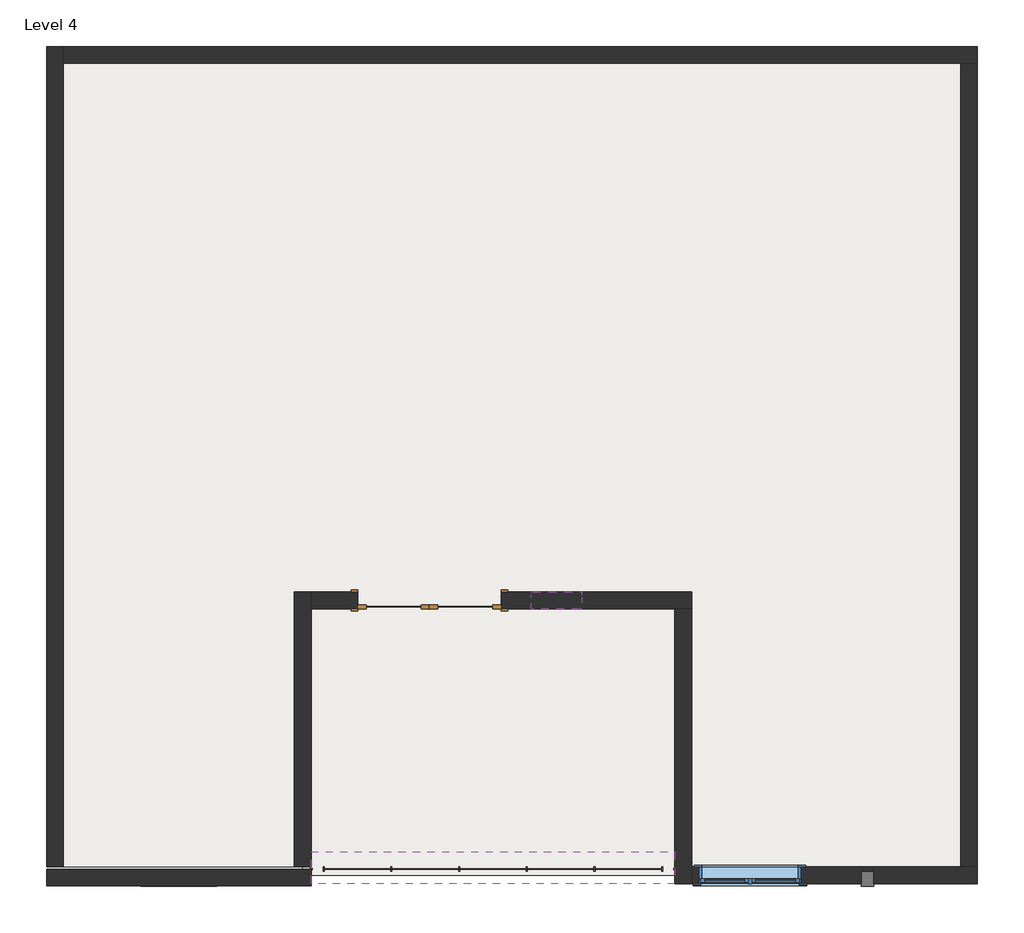
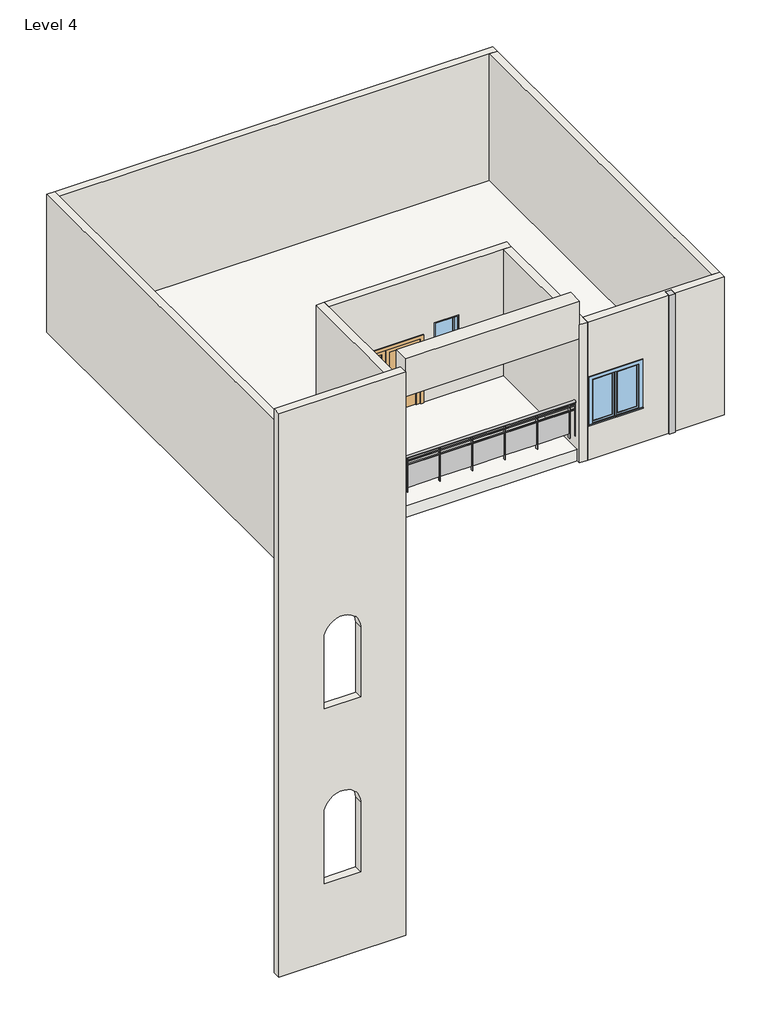
# One storey: 9 walls, 2 windows, 1 door, 1 proxy, 1 railing, 1 roof.
"""IFC4 building model written with IfcOpenShell, lengths in millimetres."""

from ifc_helpers import new_model, si_unit, point, frame, frame_2d, origin, place, context, project, spatial, polyline, circle_curve, ellipse_curve, trimmed, segment, composite_curve, outline, extrude, faceted_brep, transform, mapped, element, save
from ifc_brep_helpers import plane_surface, extruded_surface, advanced_brep
from components import door_10418eaf, walls_3_walls_2_f167fe74, window_0862ab64, window_6846e476

model = new_model("IFC4")

# Units and contexts
model_context = context("Model", 3, world=origin())
ifc_project = project(units=[si_unit("LENGTHUNIT", "METRE", prefix="MILLI")], contexts=[model_context])

# Site, building, storey
site = spatial("IfcSite", under=ifc_project)
building = spatial("IfcBuilding", under=site)
storey = spatial("IfcBuildingStorey", under=building, Name="Level 4", Elevation=10972.8)

# Proxy
placement = place(None, origin())
element("IfcBuildingElementProxy", 1, Name="Reveal", ObjectType="Reveal", at=placement, inside=storey, context=model_context, shape_type="SweptSolid", body=[
    extrude(outline(polyline([(752.5001186, 242.2810824), (752.5001186, 425.1610824), (904.9001186, 425.1610824), (904.9001186, 242.2810824), (752.5001186, 242.2810824)])), frame((0.0, 0.0, 10972.8), z_axis=(0.0, 0.0, 1.0), x_axis=(1.0, 0.0, 0.0)), (0.0, 0.0, 1.0), 3657.6),
])

# Door
door_shape = door_10418eaf(model_context)
element("IfcDoor", 2, ObjectType="Door-Double-Glass : 68\" x 80\"", at=placement, inside=storey, context=model_context, shape_type="MappedRepresentation", body=[
    mapped(door_shape, transform((-4429.0998814, 3678.7423324, 10972.8), x_axis=(-1.0, 0.0, 0.0), y_axis=(0.0, -1.0, 0.0), z_axis=(0.0, 0.0, 1.0))),
])

# Railing
element("IfcRailing", 3, ObjectType="Glass Panel - Bottom Fill", at=placement, inside=storey, context=model_context, shape_type="SolidModel", body=[
    advanced_brep(
    [(-5851.4998814, 488.6610824, 12496.8), (-5851.4998814, 412.4610824, 12496.8), (-1482.6998814, 488.6610824, 12496.8), (-1482.6998814, 412.4610824, 12496.8)],
    [
        (0, 1, ellipse_curve(frame((-5851.4998814, 450.5610824, 12496.8), z_axis=(-1.0, 0.0, 0.0), x_axis=(0.0, -1.0, 0.0)), 38.1, 28.575)),
        (1, 0, ellipse_curve(frame((-5851.4998814, 450.5610824, 12496.8), z_axis=(-1.0, 0.0, 0.0), x_axis=(0.0, -1.0, 0.0)), 38.1, 28.575)),
        (2, 3, ellipse_curve(frame((-1482.6998814, 450.5610824, 12496.8), z_axis=(1.0, 0.0, 0.0), x_axis=(0.0, -1.0, 0.0)), 38.1, 28.575)),
        (3, 2, ellipse_curve(frame((-1482.6998814, 450.5610824, 12496.8), z_axis=(1.0, 0.0, 0.0), x_axis=(0.0, -1.0, 0.0)), 38.1, 28.575)),
        (0, 2),
        (3, 1),
    ],
    [
        plane_surface(frame((-5851.4998814, 450.5610824, 12496.8), z_axis=(-1.0, 0.0, 0.0), x_axis=(0.0, 1.0, 0.0))),
        plane_surface(frame((-1482.6998814, 450.5610824, 12496.8), z_axis=(1.0, 0.0, 0.0), x_axis=(0.0, 1.0, 0.0))),
        extruded_surface(trimmed(ellipse_curve(frame((-1482.6998814, 450.5610824, 12496.8), z_axis=(-1.0, 0.0, 0.0), x_axis=(0.0, -1.0, 0.0)), 38.1, 28.575), [point((-1482.6998814, 488.6610824, 12496.8))], [point((-1482.6998814, 412.4610824, 12496.8))], True, "CARTESIAN"), (-4368.8, 0.0, 0.0), 4368.8),
        extruded_surface(trimmed(ellipse_curve(frame((-1482.6998814, 450.5610824, 12496.8), z_axis=(-1.0, 0.0, 0.0), x_axis=(0.0, -1.0, 0.0)), 38.1, 28.575), [point((-1482.6998814, 412.4610824, 12496.8))], [point((-1482.6998814, 488.6610824, 12496.8))], True, "CARTESIAN"), (-4368.8, 0.0, 0.0), 4368.8),
    ],
    [
        (0, [[1, 2]]),
        (1, [[3, 4]]),
        (2, [[-1, 5, -4, 6]]),
        (3, [[-2, -6, -3, -5]]),
    ],
),
    extrude(outline(polyline([(-5851.4998814, 437.8610824), (-5851.4998814, 463.2610824), (-1482.6998814, 463.2610824), (-1482.6998814, 437.8610824), (-5851.4998814, 437.8610824)])), frame((0.0, 0.0, 12382.5), z_axis=(0.0, 0.0, 1.0), x_axis=(1.0, 0.0, 0.0)), (0.0, 0.0, 1.0), 25.4),
    extrude(outline(polyline([(-5851.4998814, 437.8610824), (-5851.4998814, 463.2610824), (-1482.6998814, 463.2610824), (-1482.6998814, 437.8610824), (-5851.4998814, 437.8610824)])), frame((0.0, 0.0, 12280.9), z_axis=(0.0, 0.0, 1.0), x_axis=(1.0, 0.0, 0.0)), (0.0, 0.0, 1.0), 25.4),
    extrude(outline(polyline([(-1641.4498814, 425.1610824), (-1641.4498814, 475.9610824), (-1628.7498814, 475.9610824), (-1628.7498814, 425.1610824), (-1641.4498814, 425.1610824)])), frame((0.0, 0.0, 11582.4), z_axis=(0.0, 0.0, 1.0), x_axis=(1.0, 0.0, 0.0)), (0.0, 0.0, 1.0), 885.6788223),
    extrude(outline(polyline([(-2447.8998814, 457.0962394), (-1635.0998814, 457.0962394), (-1635.0998814, 450.7462394), (-2447.8998814, 450.7462394), (-2447.8998814, 457.0962394)])), frame((0.0, 0.0, 11684.0), z_axis=(0.0, 0.0, 1.0), x_axis=(1.0, 0.0, 0.0)), (0.0, 0.0, 1.0), 596.9),
    extrude(outline(polyline([(-2454.2498814, 425.1610824), (-2454.2498814, 475.9610824), (-2441.5498814, 475.9610824), (-2441.5498814, 425.1610824), (-2454.2498814, 425.1610824)])), frame((0.0, 0.0, 11582.4), z_axis=(0.0, 0.0, 1.0), x_axis=(1.0, 0.0, 0.0)), (0.0, 0.0, 1.0), 885.6788223),
    extrude(outline(polyline([(-3260.6998814, 457.0962394), (-2447.8998814, 457.0962394), (-2447.8998814, 450.7462394), (-3260.6998814, 450.7462394), (-3260.6998814, 457.0962394)])), frame((0.0, 0.0, 11684.0), z_axis=(0.0, 0.0, 1.0), x_axis=(1.0, 0.0, 0.0)), (0.0, 0.0, 1.0), 596.9),
    extrude(outline(polyline([(-3267.0498814, 425.1610824), (-3267.0498814, 475.9610824), (-3254.3498814, 475.9610824), (-3254.3498814, 425.1610824), (-3267.0498814, 425.1610824)])), frame((0.0, 0.0, 11582.4), z_axis=(0.0, 0.0, 1.0), x_axis=(1.0, 0.0, 0.0)), (0.0, 0.0, 1.0), 885.6788223),
    extrude(outline(polyline([(-4073.4998814, 457.0962394), (-3260.6998814, 457.0962394), (-3260.6998814, 450.7462394), (-4073.4998814, 450.7462394), (-4073.4998814, 457.0962394)])), frame((0.0, 0.0, 11684.0), z_axis=(0.0, 0.0, 1.0), x_axis=(1.0, 0.0, 0.0)), (0.0, 0.0, 1.0), 596.9),
    extrude(outline(polyline([(-4079.8498814, 425.1610824), (-4079.8498814, 475.9610824), (-4067.1498814, 475.9610824), (-4067.1498814, 425.1610824), (-4079.8498814, 425.1610824)])), frame((0.0, 0.0, 11582.4), z_axis=(0.0, 0.0, 1.0), x_axis=(1.0, 0.0, 0.0)), (0.0, 0.0, 1.0), 885.6788223),
    extrude(outline(polyline([(-4886.2998814, 457.0962394), (-4073.4998814, 457.0962394), (-4073.4998814, 450.7462394), (-4886.2998814, 450.7462394), (-4886.2998814, 457.0962394)])), frame((0.0, 0.0, 11684.0), z_axis=(0.0, 0.0, 1.0), x_axis=(1.0, 0.0, 0.0)), (0.0, 0.0, 1.0), 596.9),
    extrude(outline(polyline([(-4892.6498814, 425.1610824), (-4892.6498814, 475.9610824), (-4879.9498814, 475.9610824), (-4879.9498814, 425.1610824), (-4892.6498814, 425.1610824)])), frame((0.0, 0.0, 11582.4), z_axis=(0.0, 0.0, 1.0), x_axis=(1.0, 0.0, 0.0)), (0.0, 0.0, 1.0), 885.6788223),
    extrude(outline(polyline([(-5699.0998814, 457.0962394), (-4886.2998814, 457.0962394), (-4886.2998814, 450.7462394), (-5699.0998814, 450.7462394), (-5699.0998814, 457.0962394)])), frame((0.0, 0.0, 11684.0), z_axis=(0.0, 0.0, 1.0), x_axis=(1.0, 0.0, 0.0)), (0.0, 0.0, 1.0), 596.9),
    extrude(outline(polyline([(-5705.4498814, 425.1610824), (-5705.4498814, 475.9610824), (-5692.7498814, 475.9610824), (-5692.7498814, 425.1610824), (-5705.4498814, 425.1610824)])), frame((0.0, 0.0, 11582.4), z_axis=(0.0, 0.0, 1.0), x_axis=(1.0, 0.0, 0.0)), (0.0, 0.0, 1.0), 885.6788223),
    extrude(outline(polyline([(-1495.3998814, 441.0360824), (-1495.3998814, 460.0860824), (-1476.3498814, 460.0860824), (-1476.3498814, 441.0360824), (-1495.3998814, 441.0360824)])), frame((0.0, 0.0, 11582.4), z_axis=(0.0, 0.0, 1.0), x_axis=(1.0, 0.0, 0.0)), (0.0, 0.0, 1.0), 885.6788223),
    extrude(outline(polyline([(-5857.8498814, 441.0360824), (-5857.8498814, 460.0860824), (-5838.7998814, 460.0860824), (-5838.7998814, 441.0360824), (-5857.8498814, 441.0360824)])), frame((0.0, 0.0, 11582.4), z_axis=(0.0, 0.0, 1.0), x_axis=(1.0, 0.0, 0.0)), (0.0, 0.0, 1.0), 885.6788223),
])

# Roof
element("IfcRoof", 4, ObjectType="Generic - 12\"", at=placement, inside=storey, context=model_context, shape_type="SweptSolid", body=[
    extrude(outline(polyline([(-9026.4998814, 10331.1610824), (2149.5001186, 10331.1610824), (2149.5001186, 374.3610824), (-5953.0998814, 374.3610824), (-5953.0998814, 475.9610824), (-9026.4998814, 475.9610824), (-9026.4998814, 10331.1610824)])), frame((0.0, 0.0, 10972.8), z_axis=(0.0, 0.0, 1.0), x_axis=(1.0, 0.0, 0.0)), (0.0, 0.0, 1.0), 304.8),
])

# Walls
element("IfcWall", 5, ObjectType="Generic - 8\"", at=placement, inside=storey, context=model_context, shape_type="Brep", body=[
    faceted_brep([(-5851.4998814, 475.9610824, 10972.8), (-5851.4998814, 3574.7610824, 10972.8), (-5851.4998814, 3777.9610824, 10972.8), (-5851.4998814, 3777.9610824, 14630.4), (-5851.4998814, 3574.7610824, 14630.4), (-5851.4998814, 475.9610824, 14630.4), (-6054.6998814, 475.9610824, 10972.8), (-6054.6998814, 475.9610824, 14630.4), (-6054.6998814, 3777.9610824, 14630.4), (-6054.6998814, 3777.9610824, 10972.8)], [[[0, 1, 2, 3, 4, 5]], [[6, 7, 8, 9]], [[2, 1, 0, 6, 9]], [[5, 4, 3, 8, 7]], [[0, 5, 7, 6]], [[3, 2, 9, 8]]]),
])
element("IfcWall", 6, ObjectType="Generic - 8\"", at=placement, inside=storey, context=model_context, shape_type="Brep", body=[
    faceted_brep([(-5851.4998814, 3574.7610824, 10972.8), (-5292.6998814, 3574.7610824, 10972.8), (-5292.6998814, 3574.7610824, 13004.8), (-3565.4998814, 3574.7610824, 13004.8), (-3565.4998814, 3574.7610824, 10972.8), (-1482.6998814, 3574.7610824, 10972.8), (-1279.4998814, 3574.7610824, 10972.8), (-1279.4998814, 3574.7610824, 14630.4), (-1482.6998814, 3574.7610824, 14630.4), (-5851.4998814, 3574.7610824, 14630.4), (-2600.2998814, 3574.7610824, 13288.7676617), (-2600.2998814, 3574.7610824, 12679.1676617), (-3209.8998814, 3574.7610824, 12679.1676617), (-3209.8998814, 3574.7610824, 13288.7676617), (-5292.6998814, 3777.9610824, 13004.8), (-5292.6998814, 3777.9610824, 10972.8), (-5851.4998814, 3777.9610824, 10972.8), (-5851.4998814, 3777.9610824, 14630.4), (-1279.4998814, 3777.9610824, 14630.4), (-1279.4998814, 3777.9610824, 10972.8), (-3565.4998814, 3777.9610824, 10972.8), (-3565.4998814, 3777.9610824, 13004.8), (-2600.2998814, 3777.9610824, 13288.7676617), (-3209.8998814, 3777.9610824, 13288.7676617), (-3209.8998814, 3777.9610824, 12679.1676617), (-2600.2998814, 3777.9610824, 12679.1676617)], [[[0, 1, 2, 3, 4, 5, 6, 7, 8, 9], [10, 11, 12, 13]], [[14, 15, 16, 17, 18, 19, 20, 21], [22, 23, 24, 25]], [[20, 19, 6, 5, 4]], [[16, 15, 1, 0]], [[9, 8, 7, 18, 17]], [[0, 9, 17, 16]], [[7, 6, 19, 18]], [[11, 10, 22, 25]], [[12, 11, 25, 24]], [[13, 12, 24, 23]], [[10, 13, 23, 22]], [[2, 1, 15, 14]], [[3, 2, 14, 21]], [[4, 3, 21, 20]]]),
])
element("IfcWall", 7, ObjectType="Generic - 8\"", at=placement, inside=storey, context=model_context, shape_type="Brep", body=[
    faceted_brep([(-1482.6998814, 3574.7610824, 10972.8), (-1482.6998814, 272.7610824, 10972.8), (-1482.6998814, 272.7610824, 14630.4), (-1482.6998814, 3574.7610824, 14630.4), (-1279.4998814, 3574.7610824, 10972.8), (-1279.4998814, 3574.7610824, 14630.4), (-1279.4998814, 475.9610824, 14630.4), (-1279.4998814, 272.7610824, 14630.4), (-1279.4998814, 272.7610824, 10972.8), (-1279.4998814, 475.9610824, 10972.8)], [[[0, 1, 2, 3]], [[4, 5, 6, 7, 8, 9]], [[1, 0, 4, 9, 8]], [[3, 2, 7, 6, 5]], [[0, 3, 5, 4]], [[2, 1, 8, 7]]]),
])
element("IfcWall", 8, ObjectType="Generic - 8\"", at=placement, inside=storey, context=model_context, shape_type="Brep", body=[
    faceted_brep([(-1279.4998814, 272.7610824, 14630.4), (-1279.4998814, 272.7610824, 10972.8), (752.5001186, 272.7610824, 10972.8), (752.5001186, 272.7610824, 14630.4), (-1190.5998814, 272.7610824, 11887.2), (-1190.5998814, 272.7610824, 13106.4), (28.6001186, 272.7610824, 13106.4), (28.6001186, 272.7610824, 11887.2), (2149.5001186, 272.7610824, 10972.8), (2149.5001186, 272.7610824, 14630.4), (904.9001186, 272.7610824, 14630.4), (904.9001186, 272.7610824, 10972.8), (2149.5001186, 475.9610824, 10972.8), (1946.3001186, 475.9610824, 10972.8), (-1279.4998814, 475.9610824, 10972.8), (-1279.4998814, 475.9610824, 14630.4), (1946.3001186, 475.9610824, 14630.4), (2149.5001186, 475.9610824, 14630.4), (-1190.5998814, 475.9610824, 13106.4), (-1190.5998814, 475.9610824, 11887.2), (28.6001186, 475.9610824, 11887.2), (28.6001186, 475.9610824, 13106.4), (904.9001186, 425.1610824, 10972.8), (752.5001186, 425.1610824, 10972.8), (752.5001186, 425.1610824, 14630.4), (904.9001186, 425.1610824, 14630.4)], [[[0, 1, 2, 3], [4, 5, 6, 7]], [[8, 9, 10, 11]], [[12, 13, 14, 15, 16, 17], [18, 19, 20, 21]], [[14, 13, 12, 8, 11, 22, 23, 2, 1]], [[17, 16, 15, 0, 3, 24, 25, 10, 9]], [[1, 0, 15, 14]], [[9, 8, 12, 17]], [[19, 18, 5, 4]], [[20, 19, 4, 7]], [[21, 20, 7, 6]], [[18, 21, 6, 5]], [[25, 22, 11, 10]], [[22, 25, 24, 23]], [[23, 24, 3, 2]]]),
])
element("IfcWall", 9, ObjectType="Generic - 8\"", at=placement, inside=storey, context=model_context, shape_type="Brep", body=[
    faceted_brep([(-8823.2998814, 475.9610824, 10972.8), (-8823.2998814, 10127.9610824, 10972.8), (-8823.2998814, 10331.1610824, 10972.8), (-8823.2998814, 10331.1610824, 14630.4), (-8823.2998814, 10127.9610824, 14630.4), (-8823.2998814, 475.9610824, 14630.4), (-9026.4998814, 475.9610824, 10972.8), (-9026.4998814, 475.9610824, 14630.4), (-9026.4998814, 10331.1610824, 14630.4), (-9026.4998814, 10331.1610824, 10972.8)], [[[0, 1, 2, 3, 4, 5]], [[6, 7, 8, 9]], [[2, 1, 0, 6, 9]], [[5, 4, 3, 8, 7]], [[0, 5, 7, 6]], [[3, 2, 9, 8]]]),
])
element("IfcWall", 10, ObjectType="Generic - 8\"", at=placement, inside=storey, context=model_context, shape_type="Brep", body=[
    faceted_brep([(-8823.2998814, 10127.9610824, 10972.8), (1946.3001186, 10127.9610824, 10972.8), (2149.5001186, 10127.9610824, 10972.8), (2149.5001186, 10127.9610824, 14630.4), (1946.3001186, 10127.9610824, 14630.4), (-8823.2998814, 10127.9610824, 14630.4), (-8823.2998814, 10331.1610824, 10972.8), (-8823.2998814, 10331.1610824, 14630.4), (2149.5001186, 10331.1610824, 14630.4), (2149.5001186, 10331.1610824, 10972.8)], [[[0, 1, 2, 3, 4, 5]], [[6, 7, 8, 9]], [[2, 1, 0, 6, 9]], [[5, 4, 3, 8, 7]], [[0, 5, 7, 6]], [[3, 2, 9, 8]]]),
])
element("IfcWall", 11, ObjectType="Generic - 8\"", at=placement, inside=storey, context=model_context, shape_type="SweptSolid", body=[
    extrude(outline(polyline([(1946.3001186, 475.9610824), (1946.3001186, 10127.9610824), (2149.5001186, 10127.9610824), (2149.5001186, 475.9610824), (1946.3001186, 475.9610824)])), frame((0.0, 0.0, 10972.8), z_axis=(0.0, 0.0, 1.0), x_axis=(1.0, 0.0, 0.0)), (0.0, 0.0, 1.0), 3657.6),
])
element("IfcWall", 12, ObjectType="Generic - 8\"", at=placement, inside=storey, context=model_context, shape_type="SweptSolid", body=[
    extrude(outline(polyline([(0.0, -9026.4998814), (0.0, -5851.4998814), (14935.2, -5851.4998814), (14935.2, -9026.4998814), (0.0, -9026.4998814)]), holes=[composite_curve([segment(trimmed(circle_curve(frame_2d((8568.6420702, -7438.9998814)), 457.2), [point((8568.6420702, -7896.1998814))], [point((8568.6420702, -6981.7998814))], True, "CARTESIAN"), True, "CONTINUOUS"), segment(polyline([(8568.6420702, -6981.7998814), (6720.7920702, -6981.7998814), (6720.7920702, -7896.1998814), (8568.6420702, -7896.1998814)]), True, "CONTINUOUS")], self_intersect=False), composite_curve([segment(trimmed(circle_curve(frame_2d((3935.674, -7438.9998814)), 457.2), [point((3935.674, -7896.1998814))], [point((3935.674, -6981.7998814))], True, "CARTESIAN"), True, "CONTINUOUS"), segment(polyline([(3935.674, -6981.7998814), (2087.824, -6981.7998814), (2087.824, -7896.1998814), (3935.674, -7896.1998814)]), True, "CONTINUOUS")], self_intersect=False)]), frame((0.0, 247.3610824, 0.0), z_axis=(0.0, 1.0, 0.0), x_axis=(0.0, 0.0, 1.0)), (0.0, 0.0, 1.0), 203.2),
])
walls_3_walls_2_shape = walls_3_walls_2_f167fe74(model_context)
element("IfcWall", 13, ObjectType="Walls 3 : Walls 2", at=placement, inside=storey, context=model_context, shape_type="MappedRepresentation", body=[
    mapped(walls_3_walls_2_shape, transform((0.0, 0.0, 0.0), x_axis=(1.0, 0.0, 0.0), y_axis=(0.0, 1.0, 0.0), z_axis=(0.0, 0.0, 1.0))),
])

# Windows
window_shape = window_0862ab64(model_context)
element("IfcWindow", 14, ObjectType="Casement Dbl with Trim.0001 : 48\" x 48\"", at=placement, inside=storey, context=model_context, shape_type="MappedRepresentation", body=[
    mapped(window_shape, transform((-580.9998814, 393.4110824, 10972.8), x_axis=(-1.0, 0.0, 0.0), y_axis=(0.0, -1.0, 0.0), z_axis=(0.0, 0.0, 1.0))),
])
window_2_shape = window_6846e476(model_context)
element("IfcWindow", 15, ObjectType="Fixed : 24\" x 24\"", at=placement, inside=storey, context=model_context, shape_type="MappedRepresentation", body=[
    mapped(window_2_shape, transform((-2866.9998814, 3676.3610824, 11764.7676617), x_axis=(1.0, 0.0, 0.0), y_axis=(0.0, 1.0, 0.0), z_axis=(0.0, 0.0, 1.0))),
])

save(model, "model.ifc")

# Revit data of these elements
# Type "Door-Double-Glass : 68\" x 80\""
#   Type Mark = "8"
#   Construction Type Id = "opn-d45"
#   Assembly Code = "C1020"
#   Analytic Construction = "Wood frame, double glass door "
#   W = 2' - 10"
#   Thickness = 0' - 2"
#   Thermal Resistance (R) = 1.8150 (h·ft²·°F)/BTU
#   Swing Angle [instance default] = 90.00°
#   Heat Transfer Coefficient (U) = 0.5510 BTU/(h·ft²·°F)
#   Height = 6' - 8"
#   Bottom Rail = 0' - 4"
#   Top Rail = 0' - 4"
#   Stiles = 0' - 4"
#   Trim Projection = 0' - 1"
#   Trim Width = 0' - 3"
#   Width = 5' - 8"
#   Define Thermal Properties by = 1
#   Glazing = Glass
#   Panel Material = Wood - Birch - Solid Stained Light Low Gloss
#   Trim Material = Paint - Sienna
#   Visual Light Transmittance = 0
#   Solar Heat Gain Coefficient = 0
#   Function = (empty or 0)
#   Wall Closure = (empty or 0)
# Type "Glass Panel - Bottom Fill"
#   Assembly Code = "C2010400"
#   built-in parameter 1008612 = 0.0416667 (stored number, unit not read)
#   built-in parameter 1008611 = 0.0416667 (stored number, unit not read)
#   built-in parameter 1008609 = 0.333333 (stored number, unit not read)
#   built-in parameter 1008604 = 0.166667 (stored number, unit not read)
#   built-in parameter 1008603 = 0.166667 (stored number, unit not read)
#   Railing Height = 3' - 0"
#   built-in parameter 1008630 = 2
#   built-in parameter 1008610 = 2
#   built-in parameter 1008618 = Baluster - Square : 3/4"
# Type "Generic - 12\""
#   Assembly Code = "B1020"
#   Layers, outside or top first: 1' - 0" no material (function 1)
# Type "Generic - 8\""
#   Assembly Code = "B2010"
#   Layers, outside or top first: 0' - 8" no material (function 1)
# Type "Casement Dbl with Trim.0001 : 48\" x 48\""
#   Type Mark = "14"
#   Construction Type Id = "GSP4R"
#   Assembly Code = "B2020100"
#   Analytic Construction = "1/8 in Pilkington single glazing"
#   Visual Light Transmittance = 0.9
#   Solar Heat Gain Coefficient = 0.78
#   Heat Transfer Coefficient (U) = 0.6496 BTU/(h·ft²·°F)
#   Height = 4' - 0"
#   Default Sill Height = 3' - 0"
#   Trim Projection - Ext. = 0' - 0 1/2"
#   Trim Projection - Int. = 0' - 0 3/4"
#   Trim Width - Exterior = 0' - 3 1/2"
#   Trim Width - Interior = 0' - 3 1/2"
#   Width = 4' - 0"
#   Window Inset = 0' - 0 3/4"
#   Define Thermal Properties by = 1
#   Glass Pane Material = Glass
#   Sash Material = Sash
#   Trim Exterior Material = Trim
#   Trim Interior Material = Trim
#   Wall Closure = (empty or 0)
# Type "Fixed : 24\" x 24\""
#   Type Mark = "3"
#   Construction Type Id = "GSP4R"
#   Assembly Code = "B2020100"
#   Analytic Construction = "1/8 in Pilkington single glazing"
#   Visual Light Transmittance = 0.9
#   Solar Heat Gain Coefficient = 0.78
#   Heat Transfer Coefficient (U) = 0.6496 BTU/(h·ft²·°F)
#   Height = 2' - 0"
#   Default Sill Height = 3' - 0"
#   Width = 2' - 0"
#   Window Inset = 0' - 0 3/4"
#   Define Thermal Properties by = 1
#   Glass Pane Material = Glass
#   Sash Material = Sash
#   Wall Closure = (empty or 0)
# Element 2 (IfcDoor, "Door-Double-Glass : 68\" x 80\"")
#   Swing Angle = 90.00°
#   Phase Created = New Construction
#   Materials on its faces: "Wood - Birch - Solid Stained Light Low Gloss", "Paint - Sienna", "Glass"
# Element 3 (IfcRailing, "Glass Panel - Bottom Fill")
#   built-in parameter 1008621 = 2 (stored number, unit not read)
#   Phase Created = New Construction
#   Materials on its faces: "Glass"
# Element 4 (IfcRoof, "Generic - 12\"")
#   built-in parameter 1001705 = 37 (stored number, unit not read)
#   built-in parameter 1001710 = 33615
#   Phase Created = New Construction
#   Materials on its faces: "Default Roof"
# Elements 5, 6, 7, 8, 9, 10, 11 (IfcWall, "Generic - 8\"")
#   Top Offset = 0' - 0"
#   Base Offset = 0' - 0"
#   Unconnected Height = 12' - 0"
#   wall height = 12' - 0"
#   Phase Created = New Construction
#   Base Constraint = Level 4
#   Materials on its faces: "Default Wall"
# Element 12 (IfcWall, "Generic - 8\"")
#   built-in parameter 1001111 = -36' - 0"
#   Top Offset = 1' - 0"
#   Base Offset = -36' - 0"
#   wall height = 49' - 0"
#   Phase Created = New Construction
#   Base Constraint = Level 4
#   Top Constraint = Level 5
#   Materials on its faces: "Default Wall"
# Element 13 (IfcWall, "Walls 3 : Walls 2")
#   Phase Created = New Construction
#   Materials on its faces: "Default Wall"
# Element 14 (IfcWindow, "Casement Dbl with Trim.0001 : 48\" x 48\"")
#   Mark = "3"
#   Phase Created = New Construction
#   Materials on its faces: "Sash", "Trim", "Glass"
# Element 15 (IfcWindow, "Fixed : 24\" x 24\"")
#   Mark = "6"
#   Phase Created = New Construction
#   Materials on its faces: "Sash", "Glass"
# Materials
#   "Glass": class "Glass", colour RGB 0 128 192, transparency 0.75, Description = "Soda Lime Glass", Cost = 0
#   "Wood - Birch - Solid Stained Light Low Gloss": class "Wood", colour RGB 210 159 95, transparency 0, Cost = 0
#   "Paint - Sienna": colour RGB 118 70 51, transparency 0, Cost = 0
#   "Sash": class "Wood", colour RGB 224 178 126, transparency 0
#   "Trim": class "Wood", colour RGB 224 178 126, transparency 0
#   "Default Roof": colour RGB 88 101 114, transparency 0
#   "Default Wall": colour RGB 128 128 128, transparency 0
